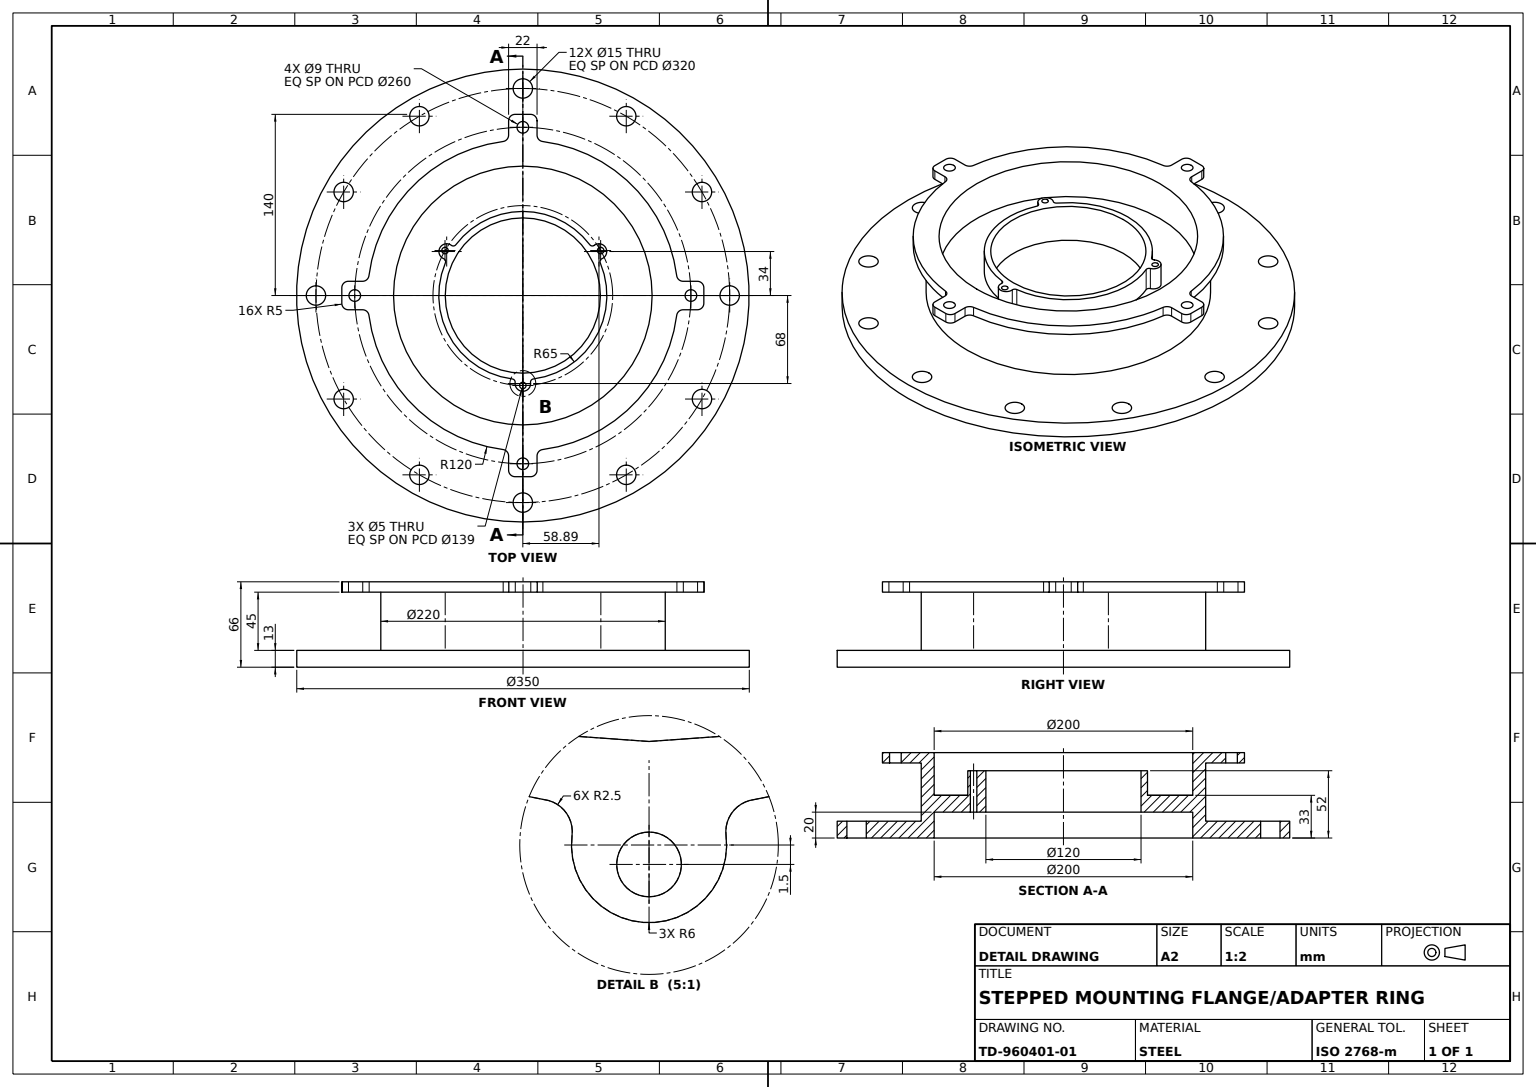
SolidWorks part; units mm, degrees
material "Plain Carbon Steel"
ref_plane "Front Plane" through (0, 0, 0) normal (0, 0, 1) x (1, 0, 0)
ref_plane "Top Plane" through (0, 0, 0) normal (0, 1, 0) x (1, 0, 0)
ref_plane "Right Plane" through (0, 0, 0) normal (1, 0, 0) x (0, 0, -1)
sketch "Base Flange Sketch" plane through (0, 0, 0) normal (0, 1, 0) x (1, 0, 0)
  circle A0 centre (0, 0) radius 175
  dimension "D1" = 350
extrude "Base Flange Ø350" add sketch "Base Flange Sketch" along normal blind 13
sketch "Hub Sketch" plane through (0, 13, 0) normal (0, 1, 0) x (1, 0, 0)
  circle A21 centre (0, 0) radius 110
  dimension "D1" = 220
extrude "Hub Boss Ø220" add sketch "Hub Sketch" along normal blind 45
sketch "Mounting Lugs Sketch" plane through (0, 58, 0) normal (0, 1, 0) x (1, 0, 0)
  line L0 (123.9718, 11) -> (135, 11)
  line L1 (0, 140) -> (6, 140)
  line L2 (11, 135) -> (11, 123.9718)
  line L4 (-11, 123.9718) -> (-11, 135)
  line L5 (-6, 140) -> (0, 140)
  line L6 (140, 6) -> (140, 0)
  line L7 (140, 0) -> (140, -6)
  line L8 (135, -11) -> (123.9718, -11)
  line L9 (11, -123.9718) -> (11, -135)
  line L10 (6, -140) -> (0, -140)
  line L11 (0, -140) -> (-6, -140)
  line L12 (-11, -135) -> (-11, -123.9718)
  line L13 (-123.9718, -11) -> (-135, -11)
  line L14 (-140, -6) -> (-140, 0)
  line L15 (-140, 0) -> (-140, 6)
  line L16 (-135, 11) -> (-123.9718, 11)
  arc A0 (-15.36, 119.0129) -> (-119.0129, 15.36) centre (0, 0) ccw
  arc A1 (6, 140) -> (11, 135) centre (6, 135) cw
  arc A2 (-11, 135) -> (-6, 140) centre (-6, 135) cw
  arc A3 (-11, 123.9718) -> (-15.36, 119.0129) centre (-16, 123.9718) cw
  arc A4 (11, 123.9718) -> (15.36, 119.0129) centre (16, 123.9718) ccw
  arc A5 (123.9718, 11) -> (119.0129, 15.36) centre (123.9718, 16) cw
  arc A6 (135, 11) -> (140, 6) centre (135, 6) cw
  arc A7 (140, -6) -> (135, -11) centre (135, -6) cw
  arc A8 (123.9718, -11) -> (119.0129, -15.36) centre (123.9718, -16) ccw
  arc A9 (11, -123.9718) -> (15.36, -119.0129) centre (16, -123.9718) cw
  arc A10 (11, -135) -> (6, -140) centre (6, -135) cw
  arc A11 (-6, -140) -> (-11, -135) centre (-6, -135) cw
  arc A12 (-11, -123.9718) -> (-15.36, -119.0129) centre (-16, -123.9718) ccw
  arc A13 (-123.9718, -11) -> (-119.0129, -15.36) centre (-123.9718, -16) cw
  arc A14 (-135, -11) -> (-140, -6) centre (-135, -6) cw
  arc A15 (-140, 6) -> (-135, 11) centre (-135, 6) cw
  arc A16 (-123.9718, 11) -> (-119.0129, 15.36) centre (-123.9718, 16) ccw
  arc A17 (119.0129, 15.36) -> (15.36, 119.0129) centre (0, 0) ccw
  arc A18 (15.36, -119.0129) -> (119.0129, -15.36) centre (0, 0) ccw
  arc A19 (-119.0129, -15.36) -> (-15.36, -119.0129) centre (0, 0) ccw
  dimension "D1" = 5
  dimension "D3" = 120
  dimension "D4" = 135
  dimension "D5" = 12
  dimension "D6" = 6
  dimension "D7" = 140
  dimension "D2" = 4
extrude "Mounting Lugs 4x" add sketch "Mounting Lugs Sketch" along normal blind 8
sketch "Bolt Holes Sketch" plane through (0, 13, 0) normal (0, 1, 0) x (1, 0, 0)
  circle A0 centre (0, 0) radius 160 construction
  circle A1 centre (0, 160) radius 7.5
  circle A2 centre (80, 138.5641) radius 7.5
  circle A3 centre (138.5641, 80) radius 7.5
  circle A4 centre (160, 0) radius 7.5
  circle A5 centre (138.5641, -80) radius 7.5
  circle A6 centre (80, -138.5641) radius 7.5
  circle A7 centre (0, -160) radius 7.5
  circle A8 centre (-80, -138.5641) radius 7.5
  circle A9 centre (-138.5641, -80) radius 7.5
  circle A10 centre (-160, 0) radius 7.5
  circle A11 centre (-138.5641, 80) radius 7.5
  circle A12 centre (-80, 138.5641) radius 7.5
  dimension "D1" = 15
  dimension "D3" = 12
  dimension "D4" = 80
  dimension "D2" = 160
  dimension "D5" = 138.5641
extrude "Bolt Holes 12xØ15" cut sketch "Bolt Holes Sketch" against normal blind 111
sketch "Upper Bore Sketch" plane through (0, 0, 0) normal (0, -1, 0) x (1, 0, 0)
  circle A0 centre (0, 0) radius 100
  dimension "D1" = 200
extrude "Upper Bore Ø200" cut sketch "Upper Bore Sketch" against normal blind 20
sketch "Inner Recess Sketch" plane through (0, 20, 0) normal (0, -1, 0) x (1, 0, 0)
  circle A0 centre (0, 0) radius 33
  dimension "D1" = 66
extrude "Inner Recess Cut" cut sketch "Inner Recess Sketch" against normal blind 13
sketch "Lower Bore Sketch" plane through (0, 33, 0) normal (0, -1, 0) x (1, 0, 0)
  circle A0 centre (0, 0) radius 100
  dimension "D1" = 200
extrude "Lower Bore Ø200" cut sketch "Lower Bore Sketch" against normal blind 53
sketch "Inner Ring Sketch" plane through (0, 20, 0) normal (0, -1, 0) x (1, 0, 0)
  arc A0 (-8.1249, 64.4902) -> (-59.9126, -25.2087) centre (0, 0) ccw
  arc A1 (5.9558, 67.2734) -> (-5.9558, 67.2734) centre (0, 68) ccw
  arc A2 (-5.9558, 67.2734) -> (-8.1249, 64.4902) centre (-8.4374, 66.9706) cw
  arc A3 (5.9558, 67.2734) -> (8.1249, 64.4902) centre (8.4374, 66.9706) ccw
  arc A4 (55.2825, -38.7946) -> (61.2384, -28.4788) centre (58.8897, -34) ccw
  arc A5 (55.2825, -38.7946) -> (51.7877, -39.2815) centre (53.7795, -40.7923) ccw
  arc A6 (61.2384, -28.4788) -> (59.9126, -25.2087) centre (62.2169, -26.1783) cw
  arc A7 (-61.2384, -28.4788) -> (-55.2825, -38.7946) centre (-58.8897, -34) ccw
  arc A8 (-61.2384, -28.4788) -> (-59.9126, -25.2087) centre (-62.2169, -26.1783) ccw
  arc A9 (-55.2825, -38.7946) -> (-51.7877, -39.2815) centre (-53.7795, -40.7923) cw
  arc A10 (59.9126, -25.2087) -> (8.1249, 64.4902) centre (0, 0) ccw
  arc A11 (-51.7877, -39.2815) -> (51.7877, -39.2815) centre (0, 0) ccw
  dimension "D1" = 2.5
  dimension "D3" = 65
  dimension "D4" = 6
  dimension "D5" = 34
  dimension "D6" = 58.8897
  dimension "D2" = 3
extrude "Inner Ring Boss" add sketch "Inner Ring Sketch" against normal blind 32
sketch "Centre Bore Sketch" plane through (0, 52, 0) normal (0, 1, 0) x (1, 0, 0)
  circle A0 centre (0, 0) radius 60
  dimension "D1" = 120
extrude "Centre Bore Ø120" cut sketch "Centre Bore Sketch" against normal blind 62
sketch "Lug Notch Sketch" plane through (0, 66, 0) normal (0, 1, 0) x (1, 0, 0)
  circle A0 centre (0, 0) radius 130 construction
  circle A1 centre (0, 130) radius 4.5
  circle A2 centre (130, 0) radius 4.5
  circle A3 centre (0, -130) radius 4.5
  circle A4 centre (-130, 0) radius 4.5
  dimension "D1" = 260
  dimension "D2" = 9
  dimension "D3" = 9
  dimension "D4" = 9
  dimension "D5" = 9
extrude "Lug Notch Cut" cut sketch "Lug Notch Sketch" against normal blind 48
sketch "Inner Ring Slots Sketch" plane through (0, 52, 0) normal (0, 1, 0) x (1, 0, 0)
  circle A0 centre (0, 0) radius 69.5 construction
  circle A1 centre (0, -69.5) radius 2.5
  circle A2 centre (-60.1888, 34.75) radius 2.5
  circle A3 centre (60.1888, 34.75) radius 2.5
  dimension "D1" = 3
  dimension "D2" = 139
  dimension "D3" = 5
  dimension "D4" = 34.75
  dimension "D5" = 60.1888
extrude "Inner Ring Slots 3x" cut sketch "Inner Ring Slots Sketch" against normal blind 48
